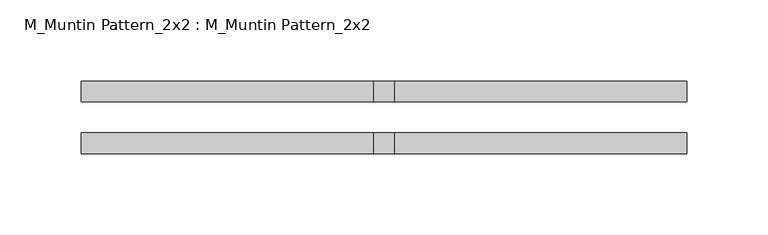
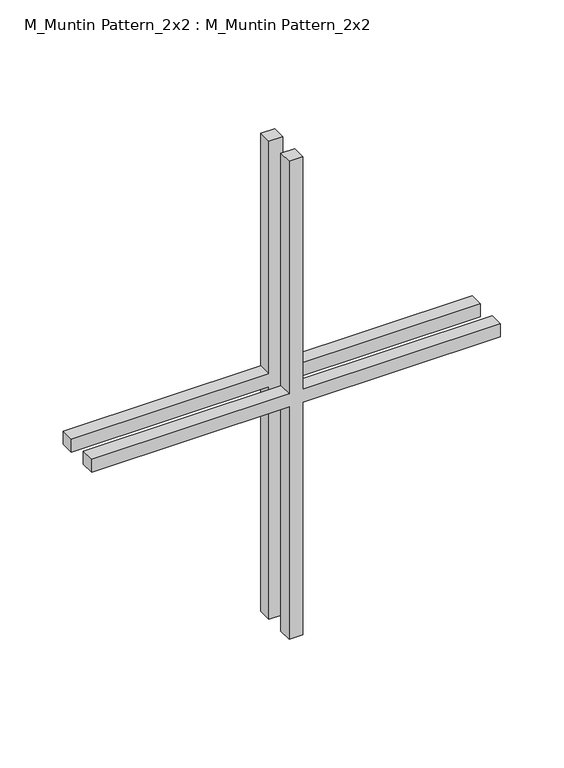
"""IFC4 building model written with IfcOpenShell, lengths in millimetres: proxy geometry, M_Muntin Pattern_2x2 : M_Muntin Pattern_2x2."""

from ifc_helpers import new_model, si_unit, frame, origin, place, context, project, spatial, polyline, outline, extrude, source, transform, mapped, element, save


def m_muntin_pattern_2x2_m_muntin_pattern_2x2_be83c6ce(model_context):
    return source(origin(), model_context, "Body", "SweptSolid", [
        extrude(outline(polyline([(236.5, -6.35), (236.5, -186.2666667), (223.8, -186.2666667), (223.8, -6.35), (0.0, -6.35), (0.0, 6.35), (223.8, 6.35), (223.8, 186.2666667), (236.5, 186.2666667), (236.5, 6.35), (460.3, 6.35), (460.3, -6.35), (236.5, -6.35)])), frame((0.0, 9.525, 0.0), z_axis=(0.0, 1.0, 0.0), x_axis=(0.0, 0.0, 1.0)), (0.0, 0.0, 1.0), 12.7),
        extrude(outline(polyline([(236.5, -6.35), (236.5, -186.2666667), (223.8, -186.2666667), (223.8, -6.35), (0.0, -6.35), (0.0, 6.35), (223.8, 6.35), (223.8, 186.2666667), (236.5, 186.2666667), (236.5, 6.35), (460.3, 6.35), (460.3, -6.35), (236.5, -6.35)])), frame((0.0, -22.225, 0.0), z_axis=(0.0, 1.0, 0.0), x_axis=(0.0, 0.0, 1.0)), (0.0, 0.0, 1.0), 12.7),
    ])


if __name__ == "__main__":
    model = new_model("IFC4")
    model_context = context("Model", 3, world=origin())
    ifc_project = project(units=[si_unit("LENGTHUNIT", "METRE", prefix="MILLI")], contexts=[model_context])
    site = spatial("IfcSite", under=ifc_project)
    building = spatial("IfcBuilding", under=site)
    placement = place(None, origin())
    m_muntin_pattern_2x2_m_muntin_pattern_2x2_shape = m_muntin_pattern_2x2_m_muntin_pattern_2x2_be83c6ce(model_context)
    element("IfcBuildingElementProxy", 1, Name="M_Muntin Pattern_2x2 : M_Muntin Pattern_2x2", ObjectType="M_Muntin Pattern_2x2 : M_Muntin Pattern_2x2", at=placement, inside=building, context=model_context, shape_type="MappedRepresentation", body=[
        mapped(m_muntin_pattern_2x2_m_muntin_pattern_2x2_shape, transform((0.0, 0.0, 0.0), x_axis=(1.0, 0.0, 0.0), y_axis=(0.0, 1.0, 0.0), z_axis=(0.0, 0.0, 1.0))),
    ])
    save(model, "model.ifc")

# Revit data of these elements
# Type "M_Muntin Pattern_2x2 : M_Muntin Pattern_2x2"
#   Width [instance default] = 3' - 11.24409"
#   Thickness = 0' - 0 1/2"
#   Height [instance default] = 3' - 11.24409"
#   Distance = 0' - 0 3/4"
#   Interior Material [instance default] = none
#   Exterior Material [instance default] = none
#   Default Elevation = 0
# Element 1 (IfcBuildingElementProxy, "M_Muntin Pattern_2x2 : M_Muntin Pattern_2x2")
#   Width = 1' - 2.66667"
#   Height = 1' - 6.12205"
#   Interior Material = Wood - Stained
#   Exterior Material = Clad - White
#   Materials on its faces: "Clad - White", "Wood - Stained"
# Materials
#   "Clad - White": class "Wood", colour RGB 242 242 238, transparency 0, Cost = 0
#   "Wood - Stained": class "Wood", colour RGB 224 178 126, transparency 0, Cost = 0
